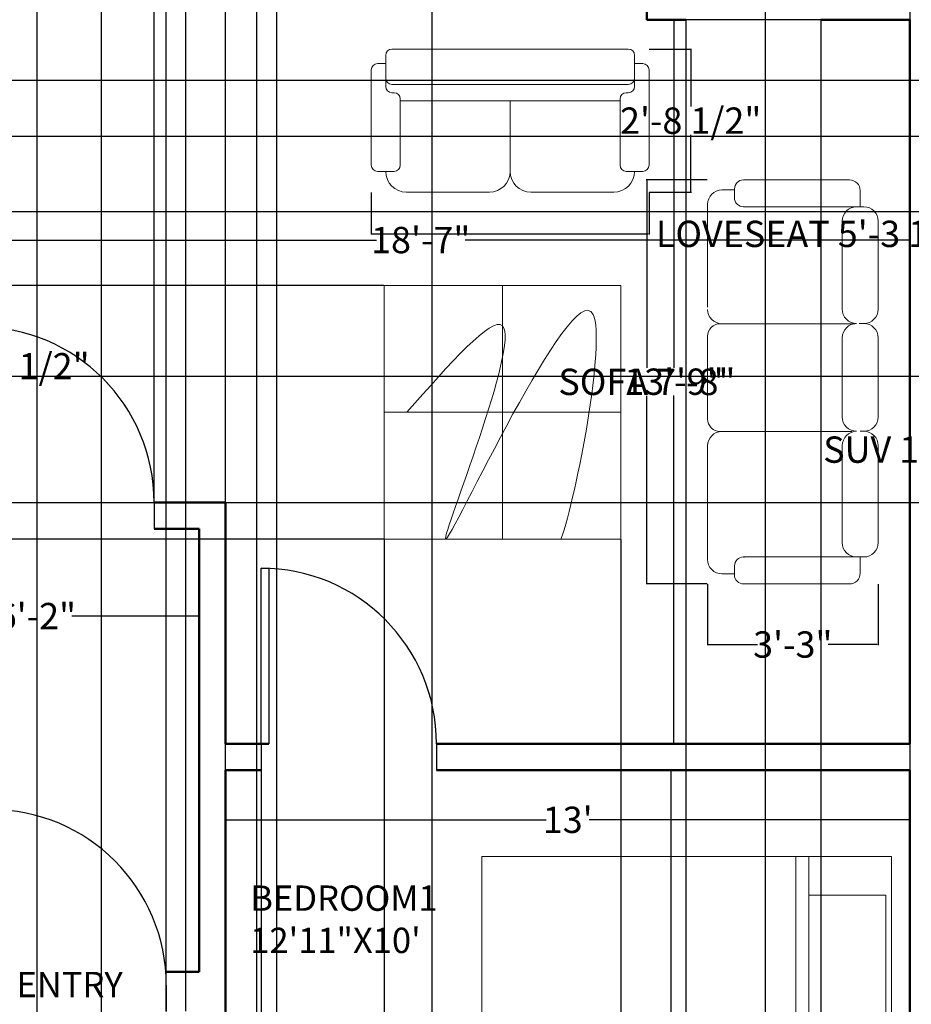
# Model space of a CAD drawing. Units: inches. Extents: x -56 to 545, y -536 to 185.
# Tile 3 of 7: x 142 to 345, y -344 to -120. Entities that reach past the tile are written whole.
import ezdxf

# ---------------------------------------------------------------- set-up
doc = ezdxf.new("R2010")
doc.units = ezdxf.units.IN
doc.header["$MEASUREMENT"] = 0
for name, color, linetype, lineweight in [('A-ANNO-DIMS', 2, 'Continuous', 18), ('A-AREA-IDEN', 4, 'Continuous', 25), ('A-DOOR', 4, 'Continuous', 25), ('A-FURN', 8, 'Continuous', 18), ('A-WALL', 7, 'Continuous', 50)]:
    doc.layers.add(name, color=color, linetype=linetype, lineweight=lineweight)
doc.styles.get("Standard").update_dxf_attribs({"font": 'arial.ttf'})
doc.dimstyles.get("Standard").update_dxf_attribs({"dimtxt": 6, "dimasz": 0.18, "dimexe": 0.18, "dimexo": 0.0625, "dimgap": 0.09, "dimtad": 0, "dimtih": 1, "dimtoh": 1, "dimdec": 0, "dimzin": 0, "dimdsep": 46, "dimlunit": 3, "dimtxsty": 'Standard', "dimcen": 0.09, "dimclrd": 3, "dimclre": 3, "dimclrt": 3, "dimadec": 0, "dimazin": 0, "dimtfac": 1, "dimtdec": 0, "dimtofl": 0, "dimtmove": 0, "dimatfit": 3, "dimfxl": 1, "dimtolj": 1, "dimtzin": 0, "dimarcsym": 0})

# ---------------------------------------------------------------- blocks, each defined once
blk = doc.blocks.new('CAMAKING')
for points in [[(0.8635, 0), (-0.8635, 0)], [(-0.8635, -2.0147), (-0.8635, 0)], [(0.8635, 0), (0.8635, -2.0147)], [(-0.6723, -0.4077), (-0.6723, -0.0281)], [(-0.6723, -0.0281), (-0.0328, -0.0281)], [(-0.0328, -0.0281), (-0.0328, -0.4077)], [(0.6716, -0.027), (0.0319, -0.027)], [(0.0319, -0.027), (0.0319, -0.4077)], [(0.6716, -0.4686), (0.6716, -0.027)], [(0.3645, -0.4056), (-0.8635, -0.4056)], [(0.8635, -0.857), (0.3645, -0.4056)], [(0.3645, -0.4702), (0.3645, -0.4056)], [(-0.8635, -0.4702), (0.3645, -0.4702)], [(0.3645, -0.4702), (0.3645, -0.857)], [(0.4362, -0.4686), (0.6716, -0.4686)], [(0.3645, -0.857), (0.8635, -0.857)], [(0.8635, -2.0147), (-0.8635, -2.0147)]]:
    blk.add_lwpolyline(points)
blk = doc.blocks.new('A$C0876780F')
for p, q in [((0.72, 0.95), (0.23, 0.95)), ((1.32, 0.95), (0.88, 0.95)), ((1.48, 0.95), (2.02, 0.95)), ((0.15, 0.85), (0.06, 0.85)), ((0.15, 0.87), (0.15, 0.8444)), ((0.15, 0.87), (0.15, 0.85)), ((0.15, 0.21), (0.15, 0.85)), ((0.8, 0.85), (0.8, 0.87)), ((0.8, 0.87), (0.8, 0.85)), ((0.8, 0.87), (0.8, 0.8444)), ((1.4, 0.85), (1.4, 0.87)), ((1.4, 0.85), (1.4, 0.87)), ((2.1, 0.87), (2.1, 0.85)), ((2.1, 0.87), (2.1, 0.8444)), ((2.1, 0.21), (2.1, 0.85)), ((2.1, 0.85), (2.19, 0.85)), ((0, 0.79), (0, 0.21)), ((0.8011, 0.8204), (0.8011, 0.08)), ((1.4014, 0.08), (1.4014, 0.803)), ((2.25, 0.79), (2.25, 0.21)), ((0.72, 0.75), (0.23, 0.75)), ((1.32, 0.75), (0.88, 0.75)), ((1.48, 0.75), (2.02, 0.75)), ((0.15, 0.2), (0.15, 0.25)), ((2.1, 0.2), (2.1, 0.25)), ((0, 0.21), (0, 0.2)), ((2.25, 0.21), (2.25, 0.2)), ((0.05, 0.15), (0.1, 0.15)), ((0.056, 0.15), (0.056, 0.08)), ((2.2, 0.15), (2.15, 0.15)), ((2.194, 0.15), (2.194, 0.08)), ((0.8011, 0.07), (0.8011, 0.08)), ((1.4014, 0.07), (1.4014, 0.08)), ((0.136, 0), (0.7093, 0)), ((0.8711, 0), (1.3314, 0)), ((2.114, 0), (1.48, 0))]:
    blk.add_line(p, q)
for centre, radius, start, end in [((0.23, 0.87), 0.08, 90, 180), ((0.72, 0.87), 0.08, 0, 90), ((0.88, 0.87), 0.08, 90, 180), ((1.32, 0.87), 0.08, 0, 90), ((1.48, 0.87), 0.08, 90, 180), ((2.02, 0.87), 0.08, 0, 90), ((0.06, 0.79), 0.06, 90, 180), ((0.23, 0.83), 0.08, 180, 270), ((0.23, 0.83), 0.08, 180, 270), ((0.72, 0.83), 0.08, 270, 0), ((0.88, 0.83), 0.08, 180, 270), ((0.88, 0.83), 0.08, 180, 270), ((1.32, 0.83), 0.08, 270, 0), ((1.48, 0.83), 0.08, 180, 270), ((2.02, 0.83), 0.08, 270, 0), ((2.02, 0.83), 0.08, 270, 0), ((2.19, 0.79), 0.06, 0, 90), ((0.05, 0.2), 0.05, 180, 270), ((0.1, 0.2), 0.05, 270, 0), ((0.09, 0.21), 0.06, 350.5377, 0), ((2.16, 0.21), 0.06, 180, 189.4623), ((2.15, 0.2), 0.05, 180, 270), ((2.2, 0.2), 0.05, 270, 0), ((0.136, 0.08), 0.08, 180, 270), ((0.7211, 0.08), 0.08, 270, 0), ((0.8711, 0.07), 0.07, 180, 270), ((1.3314, 0.07), 0.07, 270, 0), ((1.4814, 0.08), 0.08, 180, 270), ((2.114, 0.08), 0.08, 270, 0)]:
    blk.add_arc(centre, radius, start, end)
blk = doc.blocks.new('A$C02A636C4')
for p, q in [((1.2026, 0.6692), (0.097, 0.6692)), ((0.0679, 0.6013), (0.0291, 0.6013)), ((0.0679, 0.6401), (0.0679, 0.6013)), ((0.0679, 0.5334), (0.0679, 0.6013)), ((1.2317, 0.6401), (1.2317, 0.6013)), ((1.2317, 0.6013), (1.2705, 0.6013)), ((1.2317, 0.5334), (1.2317, 0.6013)), ((0, 0.5722), (0, 0.1261)), ((1.2996, 0.5722), (1.2996, 0.1261)), ((0.0679, 0.4946), (0.0679, 0.5431)), ((1.2317, 0.4946), (1.2317, 0.5431)), ((1.2026, 0.5043), (0.097, 0.5043)), ((0.1067, 0.4655), (0.097, 0.4655)), ((1.1929, 0.4655), (1.2026, 0.4655)), ((0.1358, 0.1261), (0.1358, 0.4364)), ((1.1638, 0.4267), (0.1358, 0.4267)), ((0.6498, 0.097), (0.6498, 0.4267)), ((1.1638, 0.1261), (1.1638, 0.4364)), ((0.0291, 0.097), (0.1067, 0.097)), ((1.2705, 0.097), (1.1929, 0.097)), ((0.1649, 0), (0.5528, 0)), ((0.7468, 0), (1.1347, 0))]:
    blk.add_line(p, q)
for centre, radius, start, end in [((0.097, 0.6401), 0.0291, 90, 180), ((1.2026, 0.6401), 0.0291, 0, 90), ((0.0291, 0.5722), 0.0291, 90, 180), ((1.2705, 0.5722), 0.0291, 0, 90), ((0.097, 0.5334), 0.0291, 180, 270), ((1.2026, 0.5334), 0.0291, 270, 0), ((0.097, 0.4946), 0.0291, 180, 270), ((0.1067, 0.4364), 0.0291, 0, 90), ((1.1929, 0.4364), 0.0291, 90, 180), ((1.2026, 0.4946), 0.0291, 270, 0), ((0.0291, 0.1261), 0.0291, 180, 270), ((0.1649, 0.097), 0.097, 180, 270), ((0.1067, 0.1261), 0.0291, 270, 0), ((0.5528, 0.097), 0.097, 270, 0), ((0.7468, 0.097), 0.097, 180, 270), ((1.1347, 0.097), 0.097, 270, 0), ((1.1929, 0.1261), 0.0291, 180, 270), ((1.2705, 0.1261), 0.0291, 270, 0)]:
    blk.add_arc(centre, radius, start, end)
blk = doc.blocks.new('*U7')
for p, q in [((0, 0), (0, -6)), ((40, 0), (40, -6))]:
    blk.add_line(p, q)
blk.add_lwpolyline([(0, 0), (0, 40), (1.75, 40), (1.75, 0)], close=True)
blk.add_arc((0, 0), 40, 0, 90)
blk = doc.blocks.new('*D13')
at = {"layer": 'A-ANNO-DIMS', "color": 0, "lineweight": -2, "transparency": 16777216}
for p, q in [((189.03, -302.11), (189.03, -302)), ((189.21, -302.18), (262.14, -302.18)), ((344.85, -302.18), (271.93, -302.18)), ((345.03, -302.11), (345.03, -302))]:
    blk.add_line(p, q, dxfattribs=at)
at = {"layer": 'A-ANNO-DIMS', "color": 0, "transparency": 16777216}
for points in [[(189.21, -302.15), (189.21, -302.21), (189.03, -302.18)], [(344.85, -302.15), (344.85, -302.21), (345.03, -302.18)]]:
    blk.add_solid(points, dxfattribs=at)
at = {"layer": 'Defpoints', "color": 0, "transparency": 16777216}
for p in [(189.03, -302.18), (345.03, -302.18), (345.03, -302.18)]:
    blk.add_point(p, dxfattribs=at)
at = {"layer": 'A-ANNO-DIMS', "color": 0, "transparency": 16777216, "insert": (267.03, -302.18), "char_height": 6, "attachment_point": 5}
blk.add_mtext("\\A1;13'", dxfattribs=at)
blk = doc.blocks.new('*D14')
at = {"layer": 'A-ANNO-DIMS', "color": 0, "lineweight": -2, "transparency": 16777216}
for p, q in [((290.53, -291.02), (290.53, -347.69)), ((290.6, -290.84), (290.71, -290.84)), ((290.53, -410.66), (290.53, -353.99)), ((290.6, -410.84), (290.71, -410.84))]:
    blk.add_line(p, q, dxfattribs=at)
at = {"layer": 'A-ANNO-DIMS', "color": 0, "transparency": 16777216}
for points in [[(290.5, -291.02), (290.56, -291.02), (290.53, -290.84)], [(290.5, -410.66), (290.56, -410.66), (290.53, -410.84)]]:
    blk.add_solid(points, dxfattribs=at)
at = {"layer": 'Defpoints', "color": 0, "transparency": 16777216}
for p in [(290.53, -290.84), (290.53, -290.84), (290.53, -410.84)]:
    blk.add_point(p, dxfattribs=at)
at = {"layer": 'A-ANNO-DIMS', "color": 0, "transparency": 16777216, "insert": (290.53, -350.84), "char_height": 6, "attachment_point": 5}
blk.add_mtext("\\A1;10'", dxfattribs=at)
blk = doc.blocks.new('*D19')
at = {"layer": 'A-ANNO-DIMS', "color": 0, "lineweight": -2, "transparency": 16777216}
for p, q in [((108.85, -255.7), (108.85, -255.58)), ((109.03, -255.76), (137.86, -255.76)), ((182.85, -255.76), (154.03, -255.76)), ((183.03, -255.7), (183.03, -255.58))]:
    blk.add_line(p, q, dxfattribs=at)
at = {"layer": 'A-ANNO-DIMS', "color": 0, "transparency": 16777216}
for points in [[(109.03, -255.73), (109.03, -255.79), (108.85, -255.76)], [(182.85, -255.73), (182.85, -255.79), (183.03, -255.76)]]:
    blk.add_solid(points, dxfattribs=at)
at = {"layer": 'Defpoints', "color": 0, "transparency": 16777216}
for p in [(108.85, -255.76), (183.03, -255.76), (183.03, -255.76)]:
    blk.add_point(p, dxfattribs=at)
at = {"layer": 'A-ANNO-DIMS', "color": 0, "transparency": 16777216, "insert": (145.94, -255.76), "char_height": 6, "attachment_point": 5}
blk.add_mtext('\\A1;6\'-2"', dxfattribs=at)
blk = doc.blocks.new('*D32')
at = {"layer": 'A-ANNO-DIMS', "color": 0, "lineweight": -2, "transparency": 16777216}
for p, q in [((122.03, -163.65), (122.03, -170.23)), ((345.03, -163.65), (345.03, -170.23)), ((122.21, -170.05), (223.42, -170.05)), ((344.85, -170.05), (243.65, -170.05))]:
    blk.add_line(p, q, dxfattribs=at)
at = {"layer": 'A-ANNO-DIMS', "color": 0, "transparency": 16777216}
for points in [[(122.21, -170.02), (122.21, -170.08), (122.03, -170.05)], [(344.85, -170.02), (344.85, -170.08), (345.03, -170.05)]]:
    blk.add_solid(points, dxfattribs=at)
at = {"layer": 'Defpoints', "color": 0, "transparency": 16777216}
for p in [(122.03, -163.59), (345.03, -163.59), (345.03, -170.05)]:
    blk.add_point(p, dxfattribs=at)
at = {"layer": 'A-ANNO-DIMS', "color": 0, "transparency": 16777216, "insert": (233.53, -170.05), "char_height": 6, "attachment_point": 5}
blk.add_mtext('\\A1;18\'-7"', dxfattribs=at)
blk = doc.blocks.new('*D33')
at = {"layer": 'A-ANNO-DIMS', "color": 0, "lineweight": -2, "transparency": 16777216}
for p, q in [((332.06, -119.84), (291.06, -119.84)), ((291.24, -120.02), (291.24, -199.19)), ((291.24, -284.66), (291.24, -205.5)), ((333.36, -284.84), (291.06, -284.84))]:
    blk.add_line(p, q, dxfattribs=at)
at = {"layer": 'A-ANNO-DIMS', "color": 0, "transparency": 16777216}
for points in [[(291.21, -120.02), (291.27, -120.02), (291.24, -119.84)], [(291.21, -284.66), (291.27, -284.66), (291.24, -284.84)]]:
    blk.add_solid(points, dxfattribs=at)
at = {"layer": 'Defpoints', "color": 0, "transparency": 16777216}
for p in [(291.24, -119.84), (332.12, -119.84), (333.42, -284.84)]:
    blk.add_point(p, dxfattribs=at)
at = {"layer": 'A-ANNO-DIMS', "color": 0, "transparency": 16777216, "insert": (291.24, -202.34), "char_height": 6, "attachment_point": 5}
blk.add_mtext('\\A1;13\'-9"', dxfattribs=at)
blk = doc.blocks.new('*D41')
at = {"layer": 'A-ANNO-DIMS', "color": 3, "lineweight": -2, "transparency": 16777216}
for p, q in [((298.83, -156.34), (284.9, -156.34)), ((285.08, -156.52), (285.08, -199.18)), ((285.08, -248.24), (285.08, -205.57)), ((298.83, -248.42), (284.9, -248.42))]:
    blk.add_line(p, q, dxfattribs=at)
at = {"layer": 'A-ANNO-DIMS', "color": 3, "transparency": 16777216}
for points in [[(285.05, -156.52), (285.11, -156.52), (285.08, -156.34)], [(285.05, -248.24), (285.11, -248.24), (285.08, -248.42)]]:
    blk.add_solid(points, dxfattribs=at)
at = {"layer": 'Defpoints', "color": 0, "transparency": 16777216}
for p in [(298.9, -156.34), (285.08, -248.42), (298.9, -248.42)]:
    blk.add_point(p, dxfattribs=at)
at = {"layer": 'A-ANNO-DIMS', "color": 3, "transparency": 16777216, "insert": (285.08, -202.38), "char_height": 6, "attachment_point": 5}
blk.add_mtext('\\A1;SOFA 7\'-8"', dxfattribs=at)
blk = doc.blocks.new('*D42')
at = {"layer": 'A-ANNO-DIMS', "color": 3, "lineweight": -2, "transparency": 16777216}
for p, q in [((298.9, -248.48), (298.9, -262.41)), ((337.77, -248.48), (337.77, -262.41)), ((299.08, -262.23), (310.27, -262.23)), ((337.59, -262.23), (326.4, -262.23))]:
    blk.add_line(p, q, dxfattribs=at)
at = {"layer": 'A-ANNO-DIMS', "color": 3, "transparency": 16777216}
for points in [[(299.08, -262.2), (299.08, -262.26), (298.9, -262.23)], [(337.59, -262.2), (337.59, -262.26), (337.77, -262.23)]]:
    blk.add_solid(points, dxfattribs=at)
at = {"layer": 'Defpoints', "color": 0, "transparency": 16777216}
for p in [(298.9, -248.42), (337.77, -248.42), (337.77, -262.23)]:
    blk.add_point(p, dxfattribs=at)
at = {"layer": 'A-ANNO-DIMS', "color": 3, "transparency": 16777216, "insert": (318.33, -262.23), "char_height": 6, "attachment_point": 5}
blk.add_mtext('\\A1;3\'-3"', dxfattribs=at)
blk = doc.blocks.new('*D43')
at = {"layer": 'A-ANNO-DIMS', "color": 3, "lineweight": -2, "transparency": 16777216}
for p, q in [((222.25, -159.22), (222.25, -168.83)), ((285.57, -159.22), (285.57, -168.83)), ((222.43, -168.65), (285.39, -168.65)), ((285.57, -168.65), (285.75, -168.65))]:
    blk.add_line(p, q, dxfattribs=at)
at = {"layer": 'A-ANNO-DIMS', "color": 3, "transparency": 16777216}
for points in [[(222.43, -168.62), (222.43, -168.68), (222.25, -168.65)], [(285.39, -168.62), (285.39, -168.68), (285.57, -168.65)]]:
    blk.add_solid(points, dxfattribs=at)
at = {"layer": 'Defpoints', "color": 0, "transparency": 16777216}
for p in [(222.25, -159.15), (285.57, -159.15), (285.57, -168.65)]:
    blk.add_point(p, dxfattribs=at)
at = {"layer": 'A-ANNO-DIMS', "color": 3, "transparency": 16777216, "insert": (323.96, -168.65), "char_height": 6, "attachment_point": 5}
blk.add_mtext('\\A1;LOVESEAT 5\'-3 1/2"', dxfattribs=at)
blk = doc.blocks.new('*D44')
at = {"layer": 'A-ANNO-DIMS', "color": 3, "lineweight": -2, "transparency": 16777216}
for p, q in [((285.63, -126.55), (295.24, -126.55)), ((295.06, -126.73), (295.06, -139.66)), ((295.06, -158.97), (295.06, -146.05)), ((285.63, -159.15), (295.24, -159.15))]:
    blk.add_line(p, q, dxfattribs=at)
at = {"layer": 'A-ANNO-DIMS', "color": 3, "transparency": 16777216}
for points in [[(295.03, -126.73), (295.09, -126.73), (295.06, -126.55)], [(295.03, -158.97), (295.09, -158.97), (295.06, -159.15)]]:
    blk.add_solid(points, dxfattribs=at)
at = {"layer": 'Defpoints', "color": 0, "transparency": 16777216}
for p in [(285.57, -126.55), (295.06, -126.55), (285.57, -159.15)]:
    blk.add_point(p, dxfattribs=at)
at = {"layer": 'A-ANNO-DIMS', "color": 3, "transparency": 16777216, "insert": (295.06, -142.85), "char_height": 6, "attachment_point": 5}
blk.add_mtext('\\A1;2\'-8 1/2"', dxfattribs=at)
blk = doc.blocks.new('*D45')
at = {"layer": 'A-ANNO-DIMS', "color": 3, "lineweight": -2, "transparency": 16777216}
for p, q in [((42.62, -205.02), (42.62, -198.65)), ((42.8, -198.83), (84.14, -198.83)), ((84.32, -205.02), (84.32, -198.65)), ((84.32, -198.83), (84.5, -198.83))]:
    blk.add_line(p, q, dxfattribs=at)
at = {"layer": 'A-ANNO-DIMS', "color": 3, "transparency": 16777216}
for points in [[(42.8, -198.8), (42.8, -198.86), (42.62, -198.83)], [(84.14, -198.8), (84.14, -198.86), (84.32, -198.83)]]:
    blk.add_solid(points, dxfattribs=at)
at = {"layer": 'Defpoints', "color": 0, "transparency": 16777216}
for p in [(84.32, -198.83), (42.62, -205.08), (84.32, -205.08)]:
    blk.add_point(p, dxfattribs=at)
at = {"layer": 'A-ANNO-DIMS', "color": 3, "transparency": 16777216, "insert": (121.64, -198.83), "char_height": 6, "attachment_point": 5}
blk.add_mtext('\\A1;COOKTOP 3\'-5 1/2"', dxfattribs=at)
blk = doc.blocks.new('*D47')
at = {"layer": 'A-ANNO-DIMS', "color": 3, "lineweight": -2, "transparency": 16777216}
for p, q in [((383.09, -122.58), (354.39, -122.58)), ((354.57, -122.76), (354.57, -214.63)), ((354.57, -312.89), (354.57, -221.02)), ((383.09, -313.07), (354.39, -313.07))]:
    blk.add_line(p, q, dxfattribs=at)
at = {"layer": 'A-ANNO-DIMS', "color": 3, "transparency": 16777216}
for points in [[(354.54, -122.76), (354.6, -122.76), (354.57, -122.58)], [(354.54, -312.89), (354.6, -312.89), (354.57, -313.07)]]:
    blk.add_solid(points, dxfattribs=at)
at = {"layer": 'Defpoints', "color": 0, "transparency": 16777216}
for p in [(383.15, -122.58), (354.57, -313.07), (383.15, -313.07)]:
    blk.add_point(p, dxfattribs=at)
at = {"layer": 'A-ANNO-DIMS', "color": 3, "transparency": 16777216, "insert": (354.57, -217.82), "char_height": 6, "attachment_point": 5}
blk.add_mtext('\\A1;SUV 15\'-10 1/2"', dxfattribs=at)
blk = doc.blocks.new('*D49')
at = {"layer": 'A-ANNO-DIMS', "color": 3, "lineweight": -2, "transparency": 16777216}
for p, q in [((389.1, -321.67), (363.5, -321.67)), ((363.68, -321.85), (363.68, -403.43)), ((363.68, -491.39), (363.68, -409.81)), ((389.1, -491.57), (363.5, -491.57))]:
    blk.add_line(p, q, dxfattribs=at)
at = {"layer": 'A-ANNO-DIMS', "color": 3, "transparency": 16777216}
for points in [[(363.65, -321.85), (363.71, -321.85), (363.68, -321.67)], [(363.65, -491.39), (363.71, -491.39), (363.68, -491.57)]]:
    blk.add_solid(points, dxfattribs=at)
at = {"layer": 'Defpoints', "color": 0, "transparency": 16777216}
for p in [(389.16, -321.67), (363.68, -491.57), (389.16, -491.57)]:
    blk.add_point(p, dxfattribs=at)
at = {"layer": 'A-ANNO-DIMS', "color": 3, "transparency": 16777216, "insert": (363.68, -406.62), "char_height": 6, "attachment_point": 5}
blk.add_mtext('\\A1;SEDAN 14\'-2"', dxfattribs=at)
blk = doc.blocks.new('*D59')
at = {"layer": 'A-ANNO-DIMS', "color": 3, "lineweight": -2, "transparency": 16777216}
for p, q in [((142.13, -133.66), (530.18, -133.66)), ((530, -133.84), (530, -145.47)), ((530, -163.41), (530, -151.78)), ((122.1, -163.59), (530.18, -163.59))]:
    blk.add_line(p, q, dxfattribs=at)
at = {"layer": 'A-ANNO-DIMS', "color": 3, "transparency": 16777216}
for points in [[(529.97, -133.84), (530.03, -133.84), (530, -133.66)], [(529.97, -163.41), (530.03, -163.41), (530, -163.59)]]:
    blk.add_solid(points, dxfattribs=at)
at = {"layer": 'Defpoints', "color": 0, "transparency": 16777216}
for p in [(142.07, -133.66), (530, -133.66), (122.03, -163.59)]:
    blk.add_point(p, dxfattribs=at)
at = {"layer": 'A-ANNO-DIMS', "color": 3, "transparency": 16777216, "insert": (530, -148.63), "char_height": 6, "attachment_point": 5}
blk.add_mtext('\\A1;2\'-6"', dxfattribs=at)
blk = doc.blocks.new('*D61')
at = {"layer": 'A-ANNO-DIMS', "color": 3, "lineweight": -2, "transparency": 16777216}
for p, q in [((175.54, -345.78), (175.54, 176.3)), ((175.72, 176.12), (179.85, 176.12)), ((180.03, -345.78), (180.03, 176.3)), ((180.03, 176.12), (180.21, 176.12))]:
    blk.add_line(p, q, dxfattribs=at)
at = {"layer": 'A-ANNO-DIMS', "color": 3, "transparency": 16777216}
for points in [[(175.72, 176.15), (175.72, 176.09), (175.54, 176.12)], [(179.85, 176.15), (179.85, 176.09), (180.03, 176.12)]]:
    blk.add_solid(points, dxfattribs=at)
at = {"layer": 'Defpoints', "color": 0, "transparency": 16777216}
for p in [(180.03, 176.12), (175.54, -345.84), (180.03, -345.84)]:
    blk.add_point(p, dxfattribs=at)
at = {"layer": 'A-ANNO-DIMS', "color": 3, "transparency": 16777216, "insert": (195.27, 176.12), "char_height": 6, "attachment_point": 5}
blk.add_mtext('\\A1;0\'-4 1/2"', dxfattribs=at)
blk = doc.blocks.new('*D62')
at = {"layer": 'A-ANNO-DIMS', "color": 3, "lineweight": -2, "transparency": 16777216}
for p, q in [((196.14, -419.78), (196.14, 176.3)), ((196.32, 176.12), (208.08, 176.12)), ((235.96, 176.12), (224.21, 176.12)), ((236.14, -419.78), (236.14, 176.3))]:
    blk.add_line(p, q, dxfattribs=at)
at = {"layer": 'A-ANNO-DIMS', "color": 3, "transparency": 16777216}
for points in [[(196.32, 176.15), (196.32, 176.09), (196.14, 176.12)], [(235.96, 176.15), (235.96, 176.09), (236.14, 176.12)]]:
    blk.add_solid(points, dxfattribs=at)
at = {"layer": 'Defpoints', "color": 0, "transparency": 16777216}
for p in [(236.14, 176.12), (196.14, -419.84), (236.14, -419.84)]:
    blk.add_point(p, dxfattribs=at)
at = {"layer": 'A-ANNO-DIMS', "color": 3, "transparency": 16777216, "insert": (216.14, 176.12), "char_height": 6, "attachment_point": 5}
blk.add_mtext('\\A1;3\'-4"', dxfattribs=at)
blk = doc.blocks.new('*D63')
at = {"layer": 'A-ANNO-DIMS', "color": 3, "lineweight": -2, "transparency": 16777216}
for p, q in [((189.03, -410.78), (189.03, 176.3)), ((189.21, 176.12), (195.96, 176.12)), ((196.14, -419.78), (196.14, 176.3)), ((196.14, 176.12), (196.32, 176.12))]:
    blk.add_line(p, q, dxfattribs=at)
at = {"layer": 'A-ANNO-DIMS', "color": 3, "transparency": 16777216}
for points in [[(189.21, 176.15), (189.21, 176.09), (189.03, 176.12)], [(195.96, 176.15), (195.96, 176.09), (196.14, 176.12)]]:
    blk.add_solid(points, dxfattribs=at)
at = {"layer": 'Defpoints', "color": 0, "transparency": 16777216}
for p in [(196.14, 176.12), (189.03, -410.84), (196.14, -419.84)]:
    blk.add_point(p, dxfattribs=at)
at = {"layer": 'A-ANNO-DIMS', "color": 3, "transparency": 16777216, "insert": (204.39, 176.12), "char_height": 6, "attachment_point": 5}
blk.add_mtext('\\A1;0\'-7"', dxfattribs=at)
blk = doc.blocks.new('*D64')
at = {"layer": 'A-ANNO-DIMS', "color": 3, "lineweight": -2, "transparency": 16777216}
for p, q in [((293.965457, -119.903074), (293.965457, -526.985574)), ((324.688571, -119.903074), (324.688571, -526.985574)), ((293.785457, -526.805574), (293.605457, -526.805574)), ((324.868571, -526.805574), (325.048571, -526.805574))]:
    blk.add_line(p, q, dxfattribs=at)
at = {"layer": 'A-ANNO-DIMS', "color": 3, "transparency": 16777216}
for points in [[(293.785457, -526.775574), (293.785457, -526.835574), (293.965457, -526.805574)], [(324.868571, -526.775574), (324.868571, -526.835574), (324.688571, -526.805574)]]:
    blk.add_solid(points, dxfattribs=at)
at = {"layer": 'Defpoints', "color": 0, "transparency": 16777216}
for p in [(293.965457, -119.840574), (324.688571, -119.840574), (324.688571, -526.805574)]:
    blk.add_point(p, dxfattribs=at)
at = {"layer": 'A-ANNO-DIMS', "color": 3, "transparency": 16777216, "insert": (309.327014, -526.805574), "char_height": 6, "attachment_point": 5}
blk.add_mtext('\\A1;2\'-6 1/2"', dxfattribs=at)
blk = doc.blocks.new('*D65')
at = {"layer": 'A-ANNO-DIMS', "color": 3, "lineweight": -2, "transparency": 16777216}
for p, q in [((160.69, -65.9), (160.69, -526.99)), ((200.69, -65.9), (200.69, -526.99)), ((160.87, -526.81), (172.63, -526.81)), ((200.51, -526.81), (188.76, -526.81))]:
    blk.add_line(p, q, dxfattribs=at)
at = {"layer": 'A-ANNO-DIMS', "color": 3, "transparency": 16777216}
for points in [[(160.87, -526.78), (160.87, -526.84), (160.69, -526.81)], [(200.51, -526.78), (200.51, -526.84), (200.69, -526.81)]]:
    blk.add_solid(points, dxfattribs=at)
at = {"layer": 'Defpoints', "color": 0, "transparency": 16777216}
for p in [(160.69, -65.84), (200.69, -65.84), (200.69, -526.81)]:
    blk.add_point(p, dxfattribs=at)
at = {"layer": 'A-ANNO-DIMS', "color": 3, "transparency": 16777216, "insert": (180.69, -526.81), "char_height": 6, "attachment_point": 5}
blk.add_mtext('\\A1;3\'-4"', dxfattribs=at)
blk = doc.blocks.new('*D66')
at = {"layer": 'A-ANNO-DIMS', "color": 3, "lineweight": -2, "transparency": 16777216}
for p, q in [((146.03, -65.9), (146.03, -526.99)), ((160.69, -65.9), (160.69, -526.99)), ((146.21, -526.81), (160.51, -526.81)), ((160.69, -526.81), (160.87, -526.81))]:
    blk.add_line(p, q, dxfattribs=at)
at = {"layer": 'A-ANNO-DIMS', "color": 3, "transparency": 16777216}
for points in [[(146.21, -526.78), (146.21, -526.84), (146.03, -526.81)], [(160.51, -526.78), (160.51, -526.84), (160.69, -526.81)]]:
    blk.add_solid(points, dxfattribs=at)
at = {"layer": 'Defpoints', "color": 0, "transparency": 16777216}
for p in [(146.03, -65.84), (160.69, -65.84), (160.69, -526.81)]:
    blk.add_point(p, dxfattribs=at)
at = {"layer": 'A-ANNO-DIMS', "color": 3, "transparency": 16777216, "insert": (175.65, -526.81), "char_height": 6, "attachment_point": 5}
blk.add_mtext('\\A1;1\'-2 1/2"', dxfattribs=at)
blk = doc.blocks.new('*D68')
at = {"layer": 'A-ANNO-DIMS', "color": 3, "lineweight": -2, "transparency": 16777216}
for p, q in [((172.76, -229.78), (172.76, 176.3)), ((172.94, 176.12), (188.85, 176.12)), ((189.03, -229.78), (189.03, 176.3)), ((189.03, 176.12), (189.21, 176.12))]:
    blk.add_line(p, q, dxfattribs=at)
at = {"layer": 'A-ANNO-DIMS', "color": 3, "transparency": 16777216}
for points in [[(172.94, 176.15), (172.94, 176.09), (172.76, 176.12)], [(188.85, 176.15), (188.85, 176.09), (189.03, 176.12)]]:
    blk.add_solid(points, dxfattribs=at)
at = {"layer": 'Defpoints', "color": 0, "transparency": 16777216}
for p in [(189.03, 176.12), (172.76, -229.84), (189.03, -229.84)]:
    blk.add_point(p, dxfattribs=at)
at = {"layer": 'A-ANNO-DIMS', "color": 3, "transparency": 16777216, "insert": (203.99, 176.12), "char_height": 6, "attachment_point": 5}
blk.add_mtext('\\A1;1\'-4 1/2"', dxfattribs=at)
blk = doc.blocks.new('*D69')
at = {"layer": 'A-ANNO-DIMS', "color": 3, "lineweight": -2, "transparency": 16777216}
for p, q in [((189.03, -290.9), (189.03, -526.99)), ((197.13, -290.9), (197.13, -526.99)), ((189.03, -526.81), (188.85, -526.81)), ((196.95, -526.81), (189.21, -526.81))]:
    blk.add_line(p, q, dxfattribs=at)
at = {"layer": 'A-ANNO-DIMS', "color": 3, "transparency": 16777216}
for points in [[(189.21, -526.78), (189.21, -526.84), (189.03, -526.81)], [(196.95, -526.78), (196.95, -526.84), (197.13, -526.81)]]:
    blk.add_solid(points, dxfattribs=at)
at = {"layer": 'Defpoints', "color": 0, "transparency": 16777216}
for p in [(189.03, -290.84), (197.13, -290.84), (189.03, -526.81)]:
    blk.add_point(p, dxfattribs=at)
at = {"layer": 'A-ANNO-DIMS', "color": 3, "transparency": 16777216, "insert": (180.79, -526.81), "char_height": 6, "attachment_point": 5}
blk.add_mtext('\\A1;0\'-8"', dxfattribs=at)
blk = doc.blocks.new('*D73')
at = {"layer": 'A-ANNO-DIMS', "color": 3, "lineweight": -2, "transparency": 16777216}
for p, q in [((135.38, 28.1), (135.38, -526.99)), ((140.03, 28.1), (140.03, -526.99)), ((135.56, -526.81), (139.85, -526.81)), ((140.03, -526.81), (140.21, -526.81))]:
    blk.add_line(p, q, dxfattribs=at)
at = {"layer": 'A-ANNO-DIMS', "color": 3, "transparency": 16777216}
for points in [[(135.56, -526.78), (135.56, -526.84), (135.38, -526.81)], [(139.85, -526.78), (139.85, -526.84), (140.03, -526.81)]]:
    blk.add_solid(points, dxfattribs=at)
at = {"layer": 'Defpoints', "color": 0, "transparency": 16777216}
for p in [(135.38, 28.16), (140.03, 28.16), (140.03, -526.81)]:
    blk.add_point(p, dxfattribs=at)
at = {"layer": 'A-ANNO-DIMS', "color": 3, "transparency": 16777216, "insert": (155.27, -526.81), "char_height": 6, "attachment_point": 5}
blk.add_mtext('\\A1;0\'-4 1/2"', dxfattribs=at)
blk = doc.blocks.new('*D77')
at = {"layer": 'A-ANNO-DIMS', "color": 3, "lineweight": -2, "transparency": 16777216}
for p, q in [((116.1, -201.08), (530.18, -201.08)), ((530, -201.26), (530, -212.31)), ((530, -229.66), (530, -218.61)), ((116.1, -229.84), (530.18, -229.84))]:
    blk.add_line(p, q, dxfattribs=at)
at = {"layer": 'A-ANNO-DIMS', "color": 3, "transparency": 16777216}
for points in [[(529.97, -201.26), (530.03, -201.26), (530, -201.08)], [(529.97, -229.66), (530.03, -229.66), (530, -229.84)]]:
    blk.add_solid(points, dxfattribs=at)
at = {"layer": 'Defpoints', "color": 0, "transparency": 16777216}
for p in [(116.03, -201.08), (530, -201.08), (116.03, -229.84)]:
    blk.add_point(p, dxfattribs=at)
at = {"layer": 'A-ANNO-DIMS', "color": 3, "transparency": 16777216, "insert": (530, -215.46), "char_height": 6, "attachment_point": 5}
blk.add_mtext('\\A1;2\'-5"', dxfattribs=at)
blk = doc.blocks.new('*D81')
at = {"layer": 'A-ANNO-DIMS', "color": 3, "lineweight": -2, "transparency": 16777216}
for p, q in [((345.03, 60.47), (345.03, -526.99)), ((312.03, 49.97), (312.03, -526.99)), ((312.21, -526.81), (320.42, -526.81)), ((344.85, -526.81), (336.65, -526.81))]:
    blk.add_line(p, q, dxfattribs=at)
at = {"layer": 'A-ANNO-DIMS', "color": 3, "transparency": 16777216}
for points in [[(312.21, -526.78), (312.21, -526.84), (312.03, -526.81)], [(344.85, -526.78), (344.85, -526.84), (345.03, -526.81)]]:
    blk.add_solid(points, dxfattribs=at)
at = {"layer": 'Defpoints', "color": 0, "transparency": 16777216}
for p in [(345.03, 60.53), (312.03, 50.03), (312.03, -526.81)]:
    blk.add_point(p, dxfattribs=at)
at = {"layer": 'A-ANNO-DIMS', "color": 3, "transparency": 16777216, "insert": (328.53, -526.81), "char_height": 6, "attachment_point": 5}
blk.add_mtext('\\A1;2\'-9"', dxfattribs=at)
blk = doc.blocks.new('*D83')
at = {"layer": 'A-ANNO-DIMS', "color": 3, "lineweight": -2, "transparency": 16777216}
for p, q in [((225.22, -238.28), (225.22, -526.99)), ((279.14, -238.28), (279.14, -526.99)), ((225.4, -526.81), (243.99, -526.81)), ((278.96, -526.81), (260.36, -526.81))]:
    blk.add_line(p, q, dxfattribs=at)
at = {"layer": 'A-ANNO-DIMS', "color": 3, "transparency": 16777216}
for points in [[(225.4, -526.78), (225.4, -526.84), (225.22, -526.81)], [(278.96, -526.78), (278.96, -526.84), (279.14, -526.81)]]:
    blk.add_solid(points, dxfattribs=at)
at = {"layer": 'Defpoints', "color": 0, "transparency": 16777216}
for p in [(225.22, -238.22), (279.14, -238.22), (279.14, -526.81)]:
    blk.add_point(p, dxfattribs=at)
at = {"layer": 'A-ANNO-DIMS', "color": 3, "transparency": 16777216, "insert": (252.18, -526.81), "char_height": 6, "attachment_point": 5}
blk.add_mtext('\\A1;4\'-6"', dxfattribs=at)
blk = doc.blocks.new('*D84')
at = {"layer": 'A-ANNO-DIMS', "color": 3, "lineweight": -2, "transparency": 16777216}
for p, q in [((225.15, -180.41), (-38.11, -180.41)), ((-37.93, -180.59), (-37.93, -206.16)), ((-37.93, -238.04), (-37.93, -212.47)), ((225.15, -238.22), (-38.11, -238.22))]:
    blk.add_line(p, q, dxfattribs=at)
at = {"layer": 'A-ANNO-DIMS', "color": 3, "transparency": 16777216}
for points in [[(-37.96, -180.59), (-37.9, -180.59), (-37.93, -180.41)], [(-37.96, -238.04), (-37.9, -238.04), (-37.93, -238.22)]]:
    blk.add_solid(points, dxfattribs=at)
at = {"layer": 'Defpoints', "color": 0, "transparency": 16777216}
for p in [(225.22, -180.41), (-37.93, -238.22), (225.22, -238.22)]:
    blk.add_point(p, dxfattribs=at)
at = {"layer": 'A-ANNO-DIMS', "color": 3, "transparency": 16777216, "insert": (-37.93, -209.31), "char_height": 6, "attachment_point": 5}
blk.add_mtext('\\A1;4\'-10"', dxfattribs=at)
blk = doc.blocks.new('*D86')
at = {"layer": 'A-ANNO-DIMS', "color": 3, "lineweight": -2, "transparency": 16777216}
for p, q in [((33.56, -133.66), (530.18, -133.66)), ((530, -133.84), (530, -136.81)), ((530, -146.17), (530, -143.2)), ((27.48, -146.35), (530.18, -146.35))]:
    blk.add_line(p, q, dxfattribs=at)
at = {"layer": 'A-ANNO-DIMS', "color": 3, "transparency": 16777216}
for points in [[(529.97, -133.84), (530.03, -133.84), (530, -133.66)], [(529.97, -146.17), (530.03, -146.17), (530, -146.35)]]:
    blk.add_solid(points, dxfattribs=at)
at = {"layer": 'Defpoints', "color": 0, "transparency": 16777216}
for p in [(33.5, -133.66), (27.42, -146.35), (530, -146.35)]:
    blk.add_point(p, dxfattribs=at)
at = {"layer": 'A-ANNO-DIMS', "color": 3, "transparency": 16777216, "insert": (530, -140.01), "char_height": 6, "attachment_point": 5}
blk.add_mtext('\\A1;1\'-0 1/2"', dxfattribs=at)

msp = doc.modelspace()

# ---------------------------------------------------------------- linework, layer by layer
at = {"layer": 'A-FURN'}
for p, q in [((252.18, -180.41), (252.18, -238.22)), ((225.22, -209.31), (279.14, -209.31))]:
    msp.add_line(p, q, dxfattribs=at)
msp.add_lwpolyline([(225.22, -180.41), (279.14, -180.41), (279.14, -238.22), (225.22, -238.22)], close=True, dxfattribs=at)
msp.add_open_spline([(230.39, -209.31), (240.12, -198.27), (266.5, -168.31), (216.95, -290.09), (286.29, -138.1), (269.05, -228.37), (265.49, -238.22)], degree=3, knots=[0, 0, 0, 0, 29.374629, 79.689251, 140.928736, 180.522732, 180.522732, 180.522732, 180.522732], dxfattribs=at)
at = {"layer": 'A-WALL'}
for p, q in [((285.03, -65.84), (285.03, -119.84)), ((285.03, -119.84), (293.97, -119.84)), ((324.69, -119.84), (345.03, -119.84)), ((345.03, -119.84), (345.03, -284.84)), ((172.76, -229.84), (189.03, -229.84)), ((189.03, -229.84), (189.03, -284.84)), ((172.76, -235.84), (183.03, -235.84)), ((183.03, -235.84), (183.03, -336.84)), ((189.03, -284.84), (198.88, -284.84)), ((237.13, -284.84), (345.03, -284.84)), ((189.03, -290.84), (197.13, -290.84)), ((189.03, -290.84), (189.03, -345.84)), ((237.13, -290.84), (345.03, -290.84)), ((345.03, -290.84), (345.03, -410.84)), ((175.43, -336.84), (183.03, -336.84))]:
    msp.add_line(p, q, dxfattribs=at)

# ---------------------------------------------------------------- block references
at = {"layer": 'A-DOOR'}
for p in [(132.76, -229.84), (197.13, -284.84), (135.54, -339.84)]:
    msp.add_blockref('*U7', p, dxfattribs=at)
at = {"layer": 'A-FURN', "xscale": 48.71752682720409, "yscale": 48.71752682720409, "zscale": 48.71752682720409}
msp.add_blockref('A$C02A636C4', (222.25, -159.15), dxfattribs=at)
at = {"layer": 'A-FURN', "rotation": 270}
for name, p, xscale, yscale, zscale in [('A$C0876780F', (298.9, -156.34), 40.92535895407261, 40.92535895407261, 40.92535895407261), ('CAMAKING', (340.81, -350.54), 46.34928316146463, 46.34928316146463, 46.34928316146463)]:
    msp.add_blockref(name, p, dxfattribs=dict(at, xscale=xscale, yscale=yscale, zscale=zscale))

# ---------------------------------------------------------------- texts
at = {"layer": 'A-AREA-IDEN', "attachment_point": 1}
for s, insert, char_height in [('{BEDROOM1\\P12\'11"X10\'}', (194.68, -317.15), 5.7723), ('{ENTRY}', (141.39, -336.84), 5.772)]:
    msp.add_mtext_dynamic_manual_height_columns(s, width=1091.0728, gutter_width=28.86, heights=[0], dxfattribs=dict(at, insert=insert, char_height=char_height))

# ---------------------------------------------------------------- dimensions: what is measured, and where the dimension line sits
at = {"layer": 'A-ANNO-DIMS'}
for base, p1, p2, override, picture, middle in [((189.03, 176.12), (172.76, -229.84), (189.03, -229.84), {"dimdec": 1, "dimlfac": 1, "dimrnd": 0, "dimzin": 1, "dimdsep": 46, "dimlunit": 4, "dimfrac": 2}, '*D68', (203.99, 176.12)), ((180.03, 176.12), (175.54, -345.84), (180.03, -345.84), {"dimdec": 1, "dimlfac": 1, "dimrnd": 0, "dimzin": 1, "dimdsep": 46, "dimlunit": 4, "dimfrac": 2}, '*D61', (195.27, 176.12)), ((196.14, 176.12), (189.03, -410.84), (196.14, -419.84), {"dimdec": 1, "dimlfac": 1, "dimrnd": 0, "dimzin": 1, "dimdsep": 46, "dimlunit": 4, "dimfrac": 2}, '*D63', (204.39, 176.12)), ((236.14, 176.12), (196.14, -419.84), (236.14, -419.84), {"dimdec": 1, "dimlfac": 1, "dimrnd": 0, "dimzin": 1, "dimdsep": 46, "dimlunit": 4, "dimfrac": 2}, '*D62', (216.14, 176.12)), ((312.03, -526.81), (345.03, 60.53), (312.03, 50.03), {"dimdec": 1, "dimlfac": 1, "dimrnd": 0, "dimzin": 1, "dimdsep": 46, "dimlunit": 4, "dimfrac": 2}, '*D81', (328.53, -526.81)), ((140.0343, -526.8056), (135.3838, 28.1594), (140.0343, 28.1594), {"dimdec": 1, "dimlfac": 1, "dimrnd": 0, "dimzin": 1, "dimdsep": 46, "dimlunit": 4, "dimfrac": 2}, '*D73', (155.2695, -526.8056)), ((160.69, -526.81), (146.03, -65.84), (160.69, -65.84), {"dimdec": 1, "dimlfac": 1, "dimrnd": 0, "dimzin": 1, "dimdsep": 46, "dimlunit": 4, "dimfrac": 2}, '*D66', (175.65, -526.81)), ((200.69, -526.81), (160.69, -65.84), (200.69, -65.84), {"dimdec": 1, "dimlfac": 1, "dimrnd": 0, "dimzin": 1, "dimdsep": 46, "dimlunit": 4, "dimfrac": 2}, '*D65', (180.69, -526.81)), ((324.69, -526.81), (293.97, -119.84), (324.69, -119.84), {"dimdec": 1, "dimlfac": 1, "dimrnd": 0, "dimzin": 1, "dimdsep": 46, "dimlunit": 4, "dimfrac": 2}, '*D64', (309.33, -526.81)), ((345.03, -170.05), (122.03, -163.59), (345.03, -163.59), {"dimclrd": 0, "dimclre": 0, "dimclrt": 0}, '*D32', (233.53, -170.05)), ((279.14, -526.81), (225.22, -238.22), (279.14, -238.22), {"dimdec": 1, "dimlfac": 1, "dimrnd": 0, "dimzin": 1, "dimdsep": 46, "dimlunit": 4, "dimfrac": 2}, '*D83', (252.18, -526.81)), ((337.77, -262.23), (298.9, -248.42), (337.77, -248.42), {"dimdec": 1, "dimlfac": 1, "dimrnd": 0, "dimzin": 1, "dimdsep": 46, "dimlunit": 4, "dimfrac": 2}, '*D42', (318.33, -262.23)), ((183.03, -255.76), (108.85, -255.76), (183.03, -255.76), {"dimclrd": 0, "dimclre": 0, "dimclrt": 0}, '*D19', (145.94, -255.76)), ((189.03, -526.81), (197.13, -290.84), (189.03, -290.84), {"dimdec": 1, "dimlfac": 1, "dimrnd": 0, "dimzin": 1, "dimdsep": 46, "dimlunit": 4, "dimfrac": 2}, '*D69', (180.79, -526.81)), ((345.03, -302.18), (189.03, -302.18), (345.03, -302.18), {"dimclrd": 0, "dimclre": 0, "dimclrt": 0}, '*D13', (267.03, -302.18))]:
    dim = msp.add_linear_dim(base=base, p1=p1, p2=p2, dimstyle='Standard', override=override, dxfattribs=at)
    dim.commit()
    dim.dimension.update_dxf_attribs({"geometry": picture, "text_midpoint": middle})
for base, p1, p2, override, picture, middle in [((291.24, -119.84), (333.42, -284.84), (332.12, -119.84), {"dimclrd": 0, "dimclre": 0, "dimclrt": 0}, '*D33', (291.24, -202.34)), ((295.06, -126.55), (285.57, -159.15), (285.57, -126.55), {"dimdec": 1, "dimlfac": 1, "dimrnd": 0, "dimzin": 1, "dimdsep": 46, "dimlunit": 4, "dimfrac": 2}, '*D44', (295.06, -142.85)), ((530, -146.35), (33.5, -133.66), (27.42, -146.35), {"dimdec": 1, "dimlfac": 1, "dimrnd": 0, "dimzin": 1, "dimdsep": 46, "dimlunit": 4, "dimfrac": 2}, '*D86', (530, -140.01)), ((530, -133.66), (122.03, -163.59), (142.07, -133.66), {"dimdec": 1, "dimlfac": 1, "dimrnd": 0, "dimzin": 1, "dimdsep": 46, "dimlunit": 4, "dimfrac": 2}, '*D59', (530, -148.63)), ((-37.93, -238.22), (225.22, -180.41), (225.22, -238.22), {"dimdec": 1, "dimlfac": 1, "dimrnd": 0, "dimzin": 1, "dimdsep": 46, "dimlunit": 4, "dimfrac": 2}, '*D84', (-37.93, -209.31)), ((530, -201.08), (116.03, -229.84), (116.03, -201.08), {"dimdec": 1, "dimlfac": 1, "dimrnd": 0, "dimzin": 1, "dimdsep": 46, "dimlunit": 4, "dimfrac": 2}, '*D77', (530, -215.46)), ((290.53, -290.84), (290.53, -410.84), (290.53, -290.84), {"dimclrd": 0, "dimclre": 0, "dimclrt": 0}, '*D14', (290.53, -350.84))]:
    dim = msp.add_linear_dim(base=base, p1=p1, p2=p2, angle=90, dimstyle='Standard', override=override, dxfattribs=at)
    dim.commit()
    dim.dimension.update_dxf_attribs({"geometry": picture, "text_midpoint": middle})
for base, p1, p2, text, picture, middle in [((354.57, -313.07), (383.15, -122.58), (383.15, -313.07), 'SUV <>', '*D47', (354.57, -217.82)), ((285.08, -248.42), (298.9, -156.34), (298.9, -248.42), 'SOFA <>', '*D41', (285.08, -202.38)), ((363.68, -491.57), (389.16, -321.67), (389.16, -491.57), 'SEDAN <>', '*D49', (363.68, -406.62))]:
    dim = msp.add_linear_dim(base=base, p1=p1, p2=p2, angle=270, text=text, dimstyle='Standard', override={"dimdec": 1, "dimlfac": 1, "dimrnd": 0, "dimzin": 1, "dimdsep": 46, "dimlunit": 4, "dimfrac": 2}, dxfattribs=at)
    dim.commit()
    dim.dimension.update_dxf_attribs({"geometry": picture, "text_midpoint": middle})
for base, p1, p2, text, picture, middle in [((285.57, -168.65), (222.25, -159.15), (285.57, -159.15), 'LOVESEAT <>', '*D43', (323.96, -168.65)), ((84.32, -198.83), (42.62, -205.08), (84.32, -205.08), 'COOKTOP <>', '*D45', (121.64, -198.83))]:
    dim = msp.add_linear_dim(base=base, p1=p1, p2=p2, text=text, dimstyle='Standard', override={"dimdec": 1, "dimlfac": 1, "dimrnd": 0, "dimzin": 1, "dimdsep": 46, "dimlunit": 4, "dimfrac": 2}, dxfattribs=at)
    dim.commit()
    dim.dimension.update_dxf_attribs({"geometry": picture, "text_midpoint": middle})

doc.saveas('drawing.dxf')
